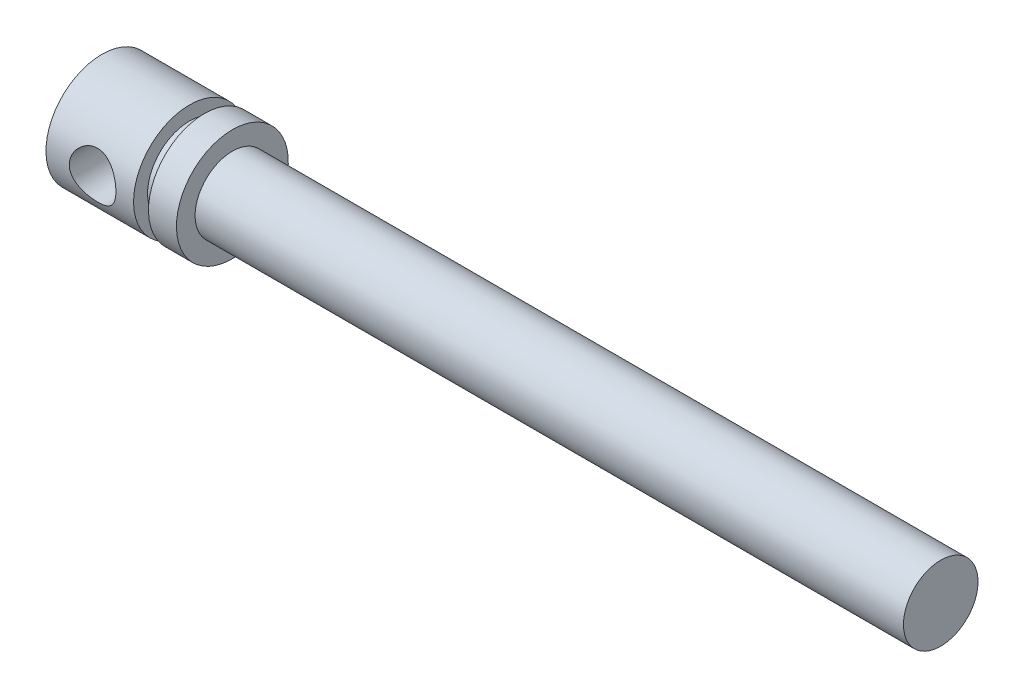
SolidWorks part; units mm, degrees
material "Plain Carbon Steel"
ref_plane "Front Plane" through (0, 0, 0) normal (0, 0, 1) x (1, 0, 0)
ref_plane "Top Plane" through (0, 0, 0) normal (0, 1, 0) x (1, 0, 0)
ref_plane "Right Plane" through (0, 0, 0) normal (1, 0, 0) x (0, 0, -1)
sketch "Screw Profile Sketch" plane through (0, 0, 0) normal (0, 0, 1) x (1, 0, 0)
  line L0 (0, 0) -> (0, 6)
  line L1 (0, 6) -> (9.4, 6)
  line L2 (9.4, 6) -> (9.4, 4.5)
  line L3 (9.4, 4.5) -> (11, 4.5)
  line L4 (11, 4.5) -> (11, 6)
  line L5 (11, 6) -> (14, 6)
  line L6 (14, 6) -> (14, 4)
  line L7 (14, 4) -> (90, 4)
  line L8 (90, 4) -> (90, 0)
  line L9 (90, 0) -> (0, 0)
  point P10 (90, 2)
  dimension "D1" = 6
  dimension "D2" = 4.5
  dimension "D3" = 4
  dimension "D4" = 90
  dimension "D5" = 14
  dimension "D6" = 1.6
  dimension "D7" = 3
revolve "Screw Body Revolve" add sketch "Screw Profile Sketch" angle 360 about L9
sketch "Cross Hole Sketch" plane through (0, 0, 0) normal (0, 0, 1) x (1, 0, 0)
  circle A0 centre (5, 0) radius 2.5
  dimension "D1" = 5
  dimension "D2" = 5
extrude "Cross Hole" cut sketch "Cross Hole Sketch" against normal through all both and the other way through all
